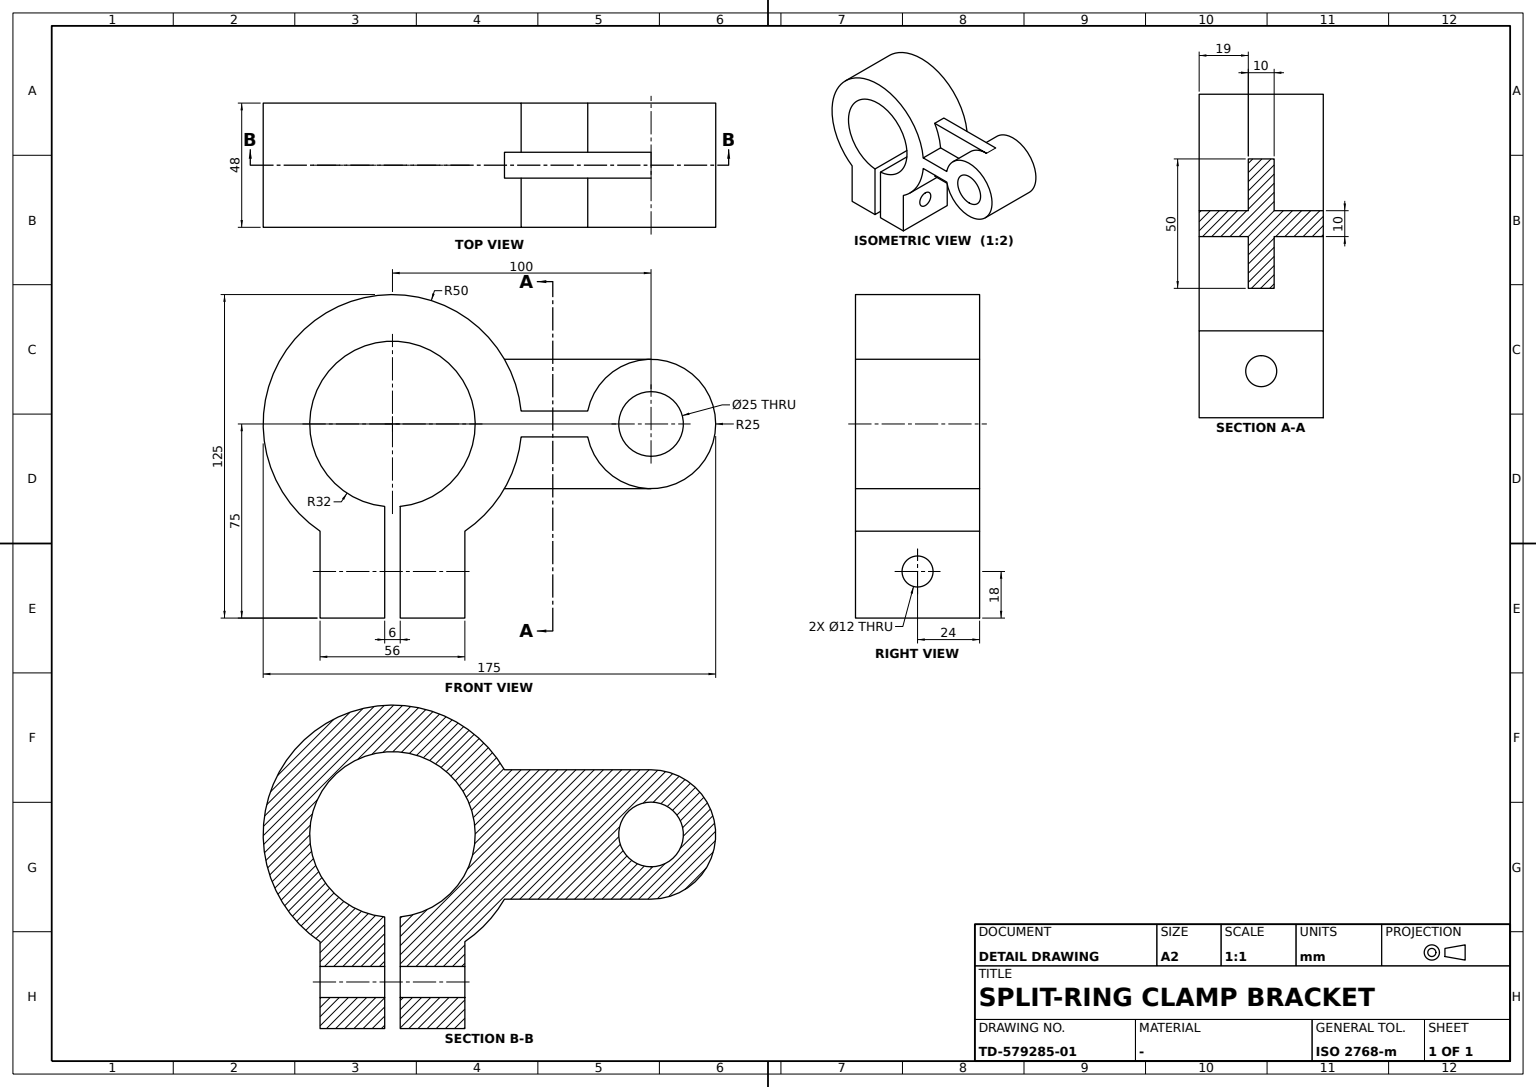
CATIA V5 part; units mm, degrees
sketch "Sketch1" plane through (0, 0, 0) normal (1, 0, 0) x (0, 1, 0)
  arc A0 (3, -31.8591) -> (-3, -31.8591) centre (0, 0) ccw
  arc A1 (28, -41.4246) -> (49.7494, -5) centre (0, 0) ccw
  line L0 (28, -75) -> (3, -75)
  line L1 (-28, -75) -> (-28, -41.4246)
  point P0 (28, 0)
  point P1 (28, -75)
  point P2 (-28, -75)
  point P3 (0, -75)
  line L2 (3, -31.8591) -> (3, -75)
  line L3 (-3, -31.8591) -> (-3, -75)
  line L4 (28, -41.4246) -> (28, -75)
  line L5 (-3, -75) -> (-28, -75)
  circle A2 centre (100, 0) radius 12.5
  point P4 (100, 0)
  arc A3 (75.5051, -5) -> (75.5051, 5) centre (100, 0) ccw
  point P5 (50, 0)
  line L6 (49.7494, 5) -> (75.5051, 5)
  point P6 (49.7494, 5)
  line L7 (49.7494, -5) -> (75.5051, -5)
  arc A4 (49.7494, 5) -> (-28, -41.4246) centre (0, 0) ccw
  dimension "radius A1" = 50
  dimension "radius A0" = 32
  dimension "length L5" = 25
  dimension "length L0" = 25
  dimension "distance L3 L2" = 6
  dimension "distance x axis L0" = 75
  dimension "radius A2" = 12.5
  dimension "distance P4 y axis" = 100
  dimension "radius A3" = 25
  dimension "distance L6 x axis" = 5
  dimension "distance L7 L6" = 10
  constraint horizontal L0 x-axis
  constraint horizontal L5 x-axis
  constraint horizontal L6 x-axis
  constraint vertical L1 y-axis
  constraint vertical L4 y-axis
  constraint coincidence L0 P3
  constraint coincidence L0 L5
  constraint coincidence P4 x-axis
  constraint coincidence P5 A1
  constraint coincidence P5 x-axis
  constraint coincidence P6 A1
  constraint coincidence A1 A4
  constraint equidistance P1 P2 P3
extrude "Pad1" add sketch "Sketch1" along normal mid plane 48
sketch "Sketch2" plane through (0, 0, 0) normal (1, 0, 0) x (0, 1, 0)
  line L0 (43.3013, 25) -> (100, 25)
  arc A0 (75.5051, -5) -> (75.5051, 5) centre (100, 0) ccw construction
  arc A1 (49.7494, 5) -> (-28, -41.4246) centre (0, 0) ccw construction
  arc A2 (49.7494, 5) -> (43.3013, 25) centre (0, 0) ccw
  point P0 (49.7494, 5)
  arc A3 (28, -41.4246) -> (49.7494, -5) centre (0, 0) ccw construction
  arc A4 (43.3013, -25) -> (49.7494, -5) centre (0, 0) ccw
  point P1 (49.7494, -5)
  line L1 (43.3013, -25) -> (100, -25)
  arc A5 (75.5051, -5) -> (75.5051, 5) centre (100, 0) ccw construction
  point P2 (43.3013, 25)
  point P3 (43.3013, -25)
  point P4 (43.3013, -25)
  point P5 (43.3013, 25)
  line L2 (75.5051, 5) -> (49.7494, 5)
  point P6 (75.5051, 5)
  point P7 (49.7494, 5)
  arc A6 (75.5051, -5) -> (75.5051, 5) centre (100, 0) ccw construction
  arc A7 (75.5051, -5) -> (100, -25) centre (100, 0) ccw
  arc A8 (100, 25) -> (75.5051, 5) centre (100, 0) ccw
  point P8 (75.5051, -5)
  point P9 (75.5051, 5)
  line L3 (49.7494, -5) -> (75.5051, -5)
  point P10 (49.7494, -5)
  point P11 (75.5051, -5)
  point P12 (100, 25)
  point P13 (100, -25)
  constraint horizontal L0 x-axis
  constraint tangency L0 A0
  constraint tangency L1 A5
  constraint symmetry L0 L1 x-axis
  constraint coincidence L0 P2
  constraint coincidence L1 P3
  constraint coincidence A3 P4
  constraint coincidence A1 P5
  constraint coincidence A6 P12
  constraint coincidence A6 P13
  constraint coincidence P0 P7
  constraint coincidence P1 P10
  constraint coincidence P2 P5
  constraint coincidence P3 P4
  constraint coincidence P6 P9
  constraint coincidence P8 P11
extrude "Pad2" add sketch "Sketch2" along normal mid plane 10
sketch "Sketch3" plane through (0, 0, 0) normal (0, 1, 0) x (-1, 0, 0)
  circle A0 centre (0, -57) radius 6
  point P0 (0, -57)
  line L0 (-24, -75) -> (-24, -41.4246) construction
  line L1 (24, -75) -> (-24, -75) construction
  dimension "radius A0" = 6
  dimension "distance P0 L0" = 24
  dimension "distance P0 L1" = 18
extrude "Pocket1" cut sketch "Sketch3" along normal mid plane 60
properties part number "8"
